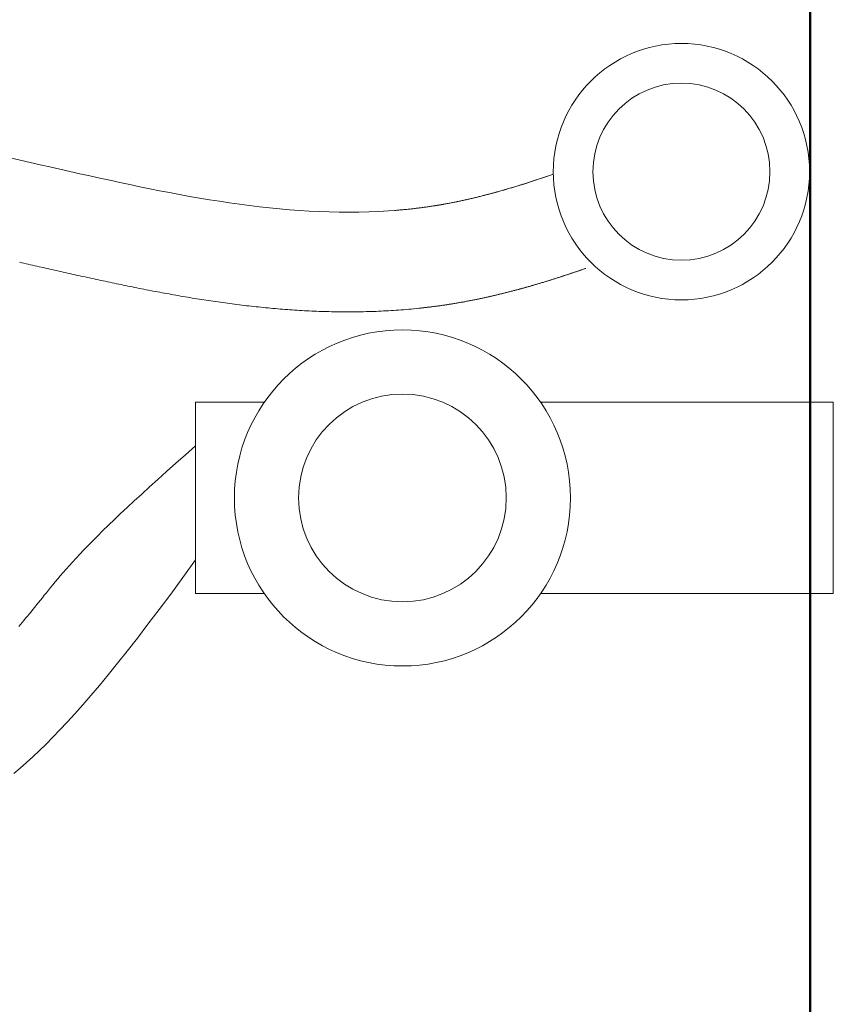
# Model space of a CAD drawing. Units: inches. Extents: x 64 to 1167, y 117 to 939.
# Tile 9 of 56: x 230.36 to 234.443, y 590.326 to 595.266. Entities that reach past the tile are written whole.
import ezdxf

# ---------------------------------------------------------------- set-up
doc = ezdxf.new("R2010")
doc.units = ezdxf.units.IN
doc.header["$MEASUREMENT"] = 0
doc.layers.add('A-FLOR-FIXT', color=8, linetype='Continuous', lineweight=18)
doc.layers.add('A-WALL', color=7, linetype='Continuous', lineweight=50)

# ---------------------------------------------------------------- blocks, each defined once
blk = doc.blocks.new('FAUCET')
for points in [[(1.4695, 2.7601), (0.0003, 2.7601), (0.0003, 1.7995), (1.4695, 1.7995)], [(2.8559, 1.7995), (3.2005, 1.7995), (3.2005, 2.7601), (2.8559, 2.7601)]]:
    blk.add_lwpolyline(points)
for points in [[(3.2005, 2.5912, 0), (3.2645, 2.6791, 0), (3.3257, 2.762, 0), (3.384, 2.8402, 0), (3.4397, 2.9138, 0), (3.493, 2.9831, 0), (3.5438, 3.0482, 0), (3.5924, 3.1094, 0), (3.639, 3.1668, 0), (3.6835, 3.2206, 0), (3.7262, 3.2711, 0), (3.7672, 3.3184, 0), (3.8067, 3.3628, 0), (3.8447, 3.4044, 0), (3.8814, 3.4435, 0), (3.9169, 3.4802, 0), (3.9514, 3.5148, 0), (3.985, 3.5473, 0), (4.0178, 3.5782, 0), (4.05, 3.6075, 0), (4.0816, 3.6354, 0), (4.1129, 3.6621, 0)], [(4.131, 0.5741, 0), (4.0812, 0.5853, 0), (4.0315, 0.5965, 0), (3.9816, 0.6078, 0), (3.9318, 0.6191, 0), (3.8819, 0.6304, 0), (3.8319, 0.6417, 0), (3.7819, 0.6529, 0), (3.7319, 0.6641, 0), (3.6819, 0.6752, 0), (3.6318, 0.6862, 0), (3.5817, 0.697, 0), (3.5316, 0.7077, 0), (3.4815, 0.7182, 0), (3.4313, 0.7284, 0), (3.3812, 0.7384, 0), (3.331, 0.7481, 0), (3.2809, 0.7575, 0), (3.2307, 0.7666, 0), (3.1806, 0.7753, 0), (3.1304, 0.7837, 0), (3.0803, 0.7916, 0), (3.0302, 0.7991, 0), (2.9801, 0.8062, 0), (2.93, 0.8128, 0), (2.88, 0.8188, 0), (2.83, 0.8244, 0), (2.78, 0.8293, 0), (2.73, 0.8337, 0), (2.6801, 0.8375, 0), (2.6302, 0.8406, 0), (2.5804, 0.8431, 0), (2.5307, 0.8449, 0), (2.4809, 0.846, 0), (2.4313, 0.8463, 0), (2.3817, 0.8458, 0), (2.3321, 0.8446, 0), (2.2827, 0.8426, 0), (2.2333, 0.8397, 0), (2.1839, 0.8359, 0), (2.1347, 0.8312, 0), (2.0855, 0.8256, 0), (2.0364, 0.8191, 0), (1.9874, 0.8116, 0), (1.9385, 0.8031, 0), (1.8897, 0.7936, 0), (1.8409, 0.7831, 0), (1.7923, 0.7717, 0), (1.7437, 0.7595, 0), (1.6952, 0.7465, 0), (1.6468, 0.7328, 0), (1.5984, 0.7185, 0), (1.55, 0.7035, 0), (1.5018, 0.6879, 0), (1.4535, 0.6719, 0), (1.4054, 0.6555, 0)], [(3.2005, 2.0185, 0), (3.2517, 2.0633, 0), (3.3003, 2.1062, 0), (3.3465, 2.1473, 0), (3.3904, 2.1866, 0), (3.4319, 2.2242, 0), (3.4713, 2.2602, 0), (3.5085, 2.2945, 0), (3.5437, 2.3273, 0), (3.5769, 2.3586, 0), (3.6083, 2.3884, 0), (3.6378, 2.4169, 0), (3.6656, 2.444, 0), (3.6917, 2.4699, 0), (3.7163, 2.4945, 0), (3.7394, 2.518, 0), (3.761, 2.5404, 0), (3.7814, 2.5617, 0), (3.8004, 2.582, 0), (3.8183, 2.6014, 0), (3.8351, 2.6199, 0), (3.8509, 2.6376, 0), (3.8657, 2.6545, 0), (3.8797, 2.6707, 0), (3.8929, 2.6862, 0), (3.9054, 2.7011, 0), (3.9172, 2.7154, 0), (3.9286, 2.7293, 0), (3.9394, 2.7427, 0), (3.9499, 2.7557, 0), (3.96, 2.7684, 0), (3.9699, 2.7808, 0), (3.9797, 2.7931, 0), (3.9893, 2.8051, 0), (3.9989, 2.8169, 0), (4.0083, 2.8285, 0), (4.0176, 2.84, 0), (4.0268, 2.8512, 0), (4.0359, 2.8623, 0), (4.0449, 2.8732, 0), (4.0538, 2.8839, 0), (4.0625, 2.8945, 0), (4.0712, 2.9048, 0), (4.0798, 2.9151, 0), (4.0883, 2.9251, 0)], [(4.0838, 1.0975, 0), (4.073, 1.0999, 0), (4.0622, 1.1023, 0), (4.0514, 1.1048, 0), (4.0406, 1.1072, 0), (4.0298, 1.1097, 0), (4.0189, 1.1121, 0), (4.0081, 1.1146, 0), (3.9972, 1.117, 0), (3.9863, 1.1195, 0), (3.9754, 1.1219, 0), (3.9645, 1.1244, 0), (3.9536, 1.1269, 0), (3.9426, 1.1293, 0), (3.9317, 1.1318, 0), (3.9207, 1.1342, 0), (3.9097, 1.1367, 0), (3.8988, 1.1392, 0), (3.8878, 1.1416, 0), (3.8767, 1.1441, 0), (3.8657, 1.1466, 0), (3.8547, 1.149, 0), (3.8437, 1.1515, 0), (3.8326, 1.154, 0), (3.8215, 1.1564, 0), (3.8104, 1.1589, 0), (3.7994, 1.1614, 0), (3.7883, 1.1638, 0), (3.7771, 1.1663, 0), (3.766, 1.1687, 0), (3.7549, 1.1712, 0), (3.7437, 1.1736, 0), (3.7325, 1.1761, 0), (3.7214, 1.1785, 0), (3.7102, 1.1809, 0), (3.699, 1.1834, 0), (3.6878, 1.1858, 0), (3.6765, 1.1882, 0), (3.6653, 1.1906, 0), (3.654, 1.193, 0), (3.6428, 1.1954, 0), (3.6315, 1.1978, 0), (3.6202, 1.2002, 0), (3.6089, 1.2026, 0), (3.5976, 1.205, 0), (3.5863, 1.2073, 0), (3.5749, 1.2097, 0), (3.5636, 1.212, 0), (3.5522, 1.2144, 0), (3.5409, 1.2167, 0), (3.5295, 1.219, 0), (3.5181, 1.2213, 0), (3.5067, 1.2236, 0), (3.4953, 1.2259, 0), (3.4838, 1.2282, 0), (3.4724, 1.2304, 0), (3.4609, 1.2327, 0), (3.4495, 1.2349, 0), (3.438, 1.2371, 0), (3.4265, 1.2394, 0), (3.415, 1.2416, 0), (3.4035, 1.2438, 0), (3.392, 1.2459, 0), (3.3804, 1.2481, 0), (3.3689, 1.2502, 0), (3.3573, 1.2524, 0), (3.3457, 1.2545, 0), (3.3342, 1.2566, 0), (3.3226, 1.2587, 0), (3.311, 1.2607, 0), (3.2993, 1.2628, 0), (3.2877, 1.2648, 0), (3.2761, 1.2669, 0), (3.2644, 1.2689, 0), (3.2527, 1.2708, 0), (3.2411, 1.2728, 0), (3.2294, 1.2748, 0), (3.2177, 1.2767, 0), (3.206, 1.2786, 0), (3.1942, 1.2805, 0), (3.1825, 1.2824, 0), (3.1708, 1.2842, 0), (3.159, 1.2861, 0), (3.1472, 1.2879, 0), (3.1354, 1.2897, 0), (3.1236, 1.2914, 0), (3.1118, 1.2932, 0), (3.1, 1.2949, 0), (3.0882, 1.2966, 0), (3.0764, 1.2983, 0), (3.0645, 1.2999, 0), (3.0526, 1.3016, 0), (3.0408, 1.3032, 0), (3.0289, 1.3048, 0), (3.017, 1.3063, 0), (3.0051, 1.3079, 0), (2.9932, 1.3094, 0), (2.9812, 1.3109, 0), (2.9693, 1.3123, 0), (2.9573, 1.3138, 0), (2.9454, 1.3152, 0), (2.9334, 1.3166, 0), (2.9214, 1.3179, 0), (2.9094, 1.3193, 0), (2.8974, 1.3206, 0), (2.8854, 1.3218, 0), (2.8733, 1.3231, 0), (2.8613, 1.3243, 0), (2.8492, 1.3255, 0), (2.8372, 1.3266, 0), (2.8251, 1.3278, 0), (2.813, 1.3289, 0), (2.8009, 1.3299, 0), (2.7888, 1.331, 0), (2.7767, 1.332, 0), (2.7645, 1.333, 0), (2.7524, 1.3339, 0), (2.7402, 1.3348, 0), (2.7281, 1.3357, 0), (2.7159, 1.3365, 0), (2.7037, 1.3374, 0), (2.6915, 1.3381, 0), (2.6793, 1.3389, 0), (2.6671, 1.3396, 0), (2.6548, 1.3403, 0), (2.6426, 1.3409, 0), (2.6303, 1.3415, 0), (2.6181, 1.3421, 0), (2.6058, 1.3427, 0), (2.5935, 1.3432, 0), (2.5812, 1.3436, 0), (2.5689, 1.3441, 0), (2.5566, 1.3445, 0), (2.5442, 1.3448, 0), (2.5319, 1.3451, 0), (2.5195, 1.3454, 0), (2.5072, 1.3457, 0), (2.4948, 1.3459, 0), (2.4824, 1.346, 0), (2.47, 1.3462, 0), (2.4576, 1.3462, 0), (2.4452, 1.3463, 0), (2.4328, 1.3463, 0), (2.4203, 1.3463, 0), (2.4079, 1.3462, 0), (2.3954, 1.3461, 0), (2.3829, 1.3459, 0), (2.3704, 1.3457, 0), (2.3579, 1.3455, 0), (2.3454, 1.3452, 0), (2.3329, 1.3449, 0), (2.3204, 1.3445, 0), (2.3079, 1.3441, 0), (2.2953, 1.3436, 0), (2.2828, 1.3431, 0), (2.2702, 1.3425, 0), (2.2576, 1.3419, 0), (2.2451, 1.3413, 0), (2.2325, 1.3406, 0), (2.2199, 1.3398, 0), (2.2073, 1.339, 0), (2.1946, 1.3382, 0), (2.182, 1.3373, 0), (2.1694, 1.3363, 0), (2.1567, 1.3354, 0), (2.1441, 1.3343, 0), (2.1314, 1.3332, 0), (2.1188, 1.3321, 0), (2.1061, 1.3309, 0), (2.0934, 1.3296, 0), (2.0807, 1.3283, 0), (2.068, 1.327, 0), (2.0553, 1.3255, 0), (2.0426, 1.3241, 0), (2.0299, 1.3226, 0), (2.0172, 1.321, 0), (2.0045, 1.3194, 0), (1.9917, 1.3177, 0), (1.979, 1.3159, 0), (1.9662, 1.3141, 0), (1.9535, 1.3123, 0), (1.9407, 1.3104, 0), (1.9279, 1.3084, 0), (1.9152, 1.3064, 0), (1.9024, 1.3043, 0), (1.8896, 1.3022, 0), (1.8769, 1.3, 0), (1.8642, 1.2977, 0), (1.8515, 1.2954, 0), (1.8388, 1.2931, 0), (1.8262, 1.2907, 0), (1.8136, 1.2882, 0), (1.801, 1.2857, 0), (1.7884, 1.2832, 0), (1.7759, 1.2806, 0), (1.7634, 1.2779, 0), (1.7509, 1.2752, 0), (1.7385, 1.2725, 0), (1.726, 1.2697, 0), (1.7137, 1.2669, 0), (1.7013, 1.264, 0), (1.689, 1.2611, 0), (1.6767, 1.2582, 0), (1.6644, 1.2552, 0), (1.6521, 1.2521, 0), (1.6399, 1.2491, 0), (1.6277, 1.246, 0), (1.6156, 1.2428, 0), (1.6034, 1.2396, 0), (1.5913, 1.2364, 0), (1.5792, 1.2332, 0), (1.5672, 1.2299, 0), (1.5552, 1.2266, 0), (1.5432, 1.2232, 0), (1.5312, 1.2199, 0), (1.5193, 1.2165, 0), (1.5074, 1.213, 0), (1.4955, 1.2096, 0), (1.4837, 1.2061, 0), (1.4719, 1.2026, 0), (1.4601, 1.199, 0), (1.4483, 1.1954, 0), (1.4366, 1.1919, 0), (1.4249, 1.1882, 0), (1.4133, 1.1846, 0), (1.4016, 1.181, 0), (1.39, 1.1773, 0), (1.3784, 1.1736, 0), (1.3669, 1.1699, 0), (1.3554, 1.1661, 0), (1.3439, 1.1624, 0), (1.3325, 1.1586, 0), (1.321, 1.1548, 0), (1.3097, 1.151, 0), (1.2983, 1.1472, 0), (1.287, 1.1434, 0), (1.2757, 1.1396, 0), (1.2644, 1.1357, 0), (1.2532, 1.1319, 0), (1.242, 1.128, 0)], [(2.0792, 1.3282, 0), (2.0747, 1.3277, 0), (2.0701, 1.3272, 0), (2.0655, 1.3267, 0), (2.0609, 1.3262, 0), (2.0563, 1.3257, 0), (2.0518, 1.3251, 0), (2.0472, 1.3246, 0), (2.0426, 1.3241, 0), (2.038, 1.3235, 0), (2.0334, 1.323, 0), (2.0288, 1.3224, 0), (2.0242, 1.3219, 0), (2.0197, 1.3213, 0), (2.0151, 1.3207, 0), (2.0105, 1.3201, 0), (2.0059, 1.3195, 0), (2.0013, 1.3189, 0), (1.9967, 1.3183, 0), (1.9921, 1.3177, 0), (1.9875, 1.3171, 0), (1.9829, 1.3165, 0), (1.9783, 1.3159, 0), (1.9737, 1.3152, 0), (1.9691, 1.3146, 0), (1.9645, 1.3139, 0), (1.9599, 1.3132, 0), (1.9553, 1.3126, 0), (1.9507, 1.3119, 0), (1.9461, 1.3112, 0), (1.9415, 1.3105, 0), (1.9369, 1.3098, 0), (1.9323, 1.3091, 0), (1.9277, 1.3084, 0), (1.9231, 1.3077, 0), (1.9185, 1.3069, 0), (1.9139, 1.3062, 0), (1.9093, 1.3054, 0), (1.9047, 1.3047, 0), (1.9001, 1.3039, 0), (1.8955, 1.3032, 0), (1.8909, 1.3024, 0), (1.8863, 1.3016, 0), (1.8817, 1.3008, 0), (1.8771, 1.3, 0), (1.8725, 1.2992, 0), (1.8679, 1.2984, 0), (1.8633, 1.2976, 0), (1.8587, 1.2968, 0), (1.8541, 1.2959, 0), (1.8496, 1.2951, 0), (1.845, 1.2943, 0), (1.8404, 1.2934, 0), (1.8359, 1.2925, 0), (1.8313, 1.2917, 0), (1.8268, 1.2908, 0), (1.8222, 1.2899, 0), (1.8177, 1.289, 0), (1.8131, 1.2882, 0), (1.8086, 1.2873, 0), (1.804, 1.2863, 0), (1.7995, 1.2854, 0), (1.795, 1.2845, 0), (1.7904, 1.2836, 0), (1.7859, 1.2827, 0), (1.7814, 1.2817, 0), (1.7769, 1.2808, 0), (1.7724, 1.2798, 0), (1.7679, 1.2789, 0), (1.7634, 1.2779, 0), (1.7589, 1.277, 0), (1.7544, 1.276, 0), (1.7499, 1.275, 0), (1.7454, 1.274, 0), (1.7409, 1.273, 0), (1.7364, 1.272, 0), (1.7319, 1.271, 0), (1.7275, 1.27, 0), (1.723, 1.269, 0), (1.7185, 1.268, 0), (1.714, 1.267, 0), (1.7096, 1.266, 0), (1.7051, 1.2649, 0), (1.7007, 1.2639, 0), (1.6962, 1.2628, 0), (1.6918, 1.2618, 0), (1.6873, 1.2607, 0), (1.6829, 1.2597, 0), (1.6785, 1.2586, 0), (1.674, 1.2575, 0), (1.6696, 1.2564, 0), (1.6652, 1.2554, 0), (1.6607, 1.2543, 0), (1.6563, 1.2532, 0), (1.6519, 1.2521, 0), (1.6475, 1.251, 0), (1.6431, 1.2499, 0), (1.6387, 1.2488, 0), (1.6343, 1.2476, 0), (1.6299, 1.2465, 0), (1.6255, 1.2454, 0), (1.6211, 1.2443, 0), (1.6167, 1.2431, 0), (1.6124, 1.242, 0), (1.608, 1.2408, 0), (1.6036, 1.2397, 0), (1.5992, 1.2385, 0), (1.5949, 1.2374, 0), (1.5905, 1.2362, 0), (1.5862, 1.235, 0), (1.5818, 1.2339, 0), (1.5774, 1.2327, 0), (1.5731, 1.2315, 0), (1.5688, 1.2303, 0), (1.5644, 1.2291, 0), (1.5601, 1.2279, 0), (1.5558, 1.2267, 0), (1.5514, 1.2255, 0), (1.5471, 1.2243, 0), (1.5428, 1.2231, 0), (1.5385, 1.2219, 0), (1.5342, 1.2207, 0), (1.5298, 1.2195, 0), (1.5255, 1.2182, 0), (1.5212, 1.217, 0), (1.5169, 1.2158, 0), (1.5126, 1.2145, 0), (1.5084, 1.2133, 0), (1.5041, 1.2121, 0), (1.4998, 1.2108, 0), (1.4955, 1.2096, 0), (1.4912, 1.2083, 0), (1.487, 1.207, 0), (1.4827, 1.2058, 0), (1.4784, 1.2045, 0), (1.4742, 1.2032, 0), (1.4699, 1.202, 0), (1.4657, 1.2007, 0), (1.4614, 1.1994, 0), (1.4572, 1.1981, 0), (1.4529, 1.1969, 0), (1.4487, 1.1956, 0), (1.4445, 1.1943, 0), (1.4403, 1.193, 0), (1.436, 1.1917, 0), (1.4318, 1.1904, 0), (1.4276, 1.1891, 0), (1.4234, 1.1878, 0), (1.4192, 1.1865, 0), (1.415, 1.1851, 0), (1.4108, 1.1838, 0), (1.4066, 1.1825, 0), (1.4024, 1.1812, 0), (1.3982, 1.1799, 0), (1.394, 1.1785, 0), (1.3898, 1.1772, 0), (1.3856, 1.1759, 0), (1.3815, 1.1746, 0), (1.3773, 1.1732, 0), (1.3731, 1.1719, 0), (1.369, 1.1705, 0), (1.3648, 1.1692, 0), (1.3607, 1.1678, 0), (1.3565, 1.1665, 0), (1.3524, 1.1652, 0), (1.3482, 1.1638, 0), (1.3441, 1.1624, 0), (1.34, 1.1611, 0), (1.3358, 1.1597, 0), (1.3317, 1.1584, 0), (1.3276, 1.157, 0), (1.3235, 1.1556, 0), (1.3194, 1.1543, 0), (1.3153, 1.1529, 0), (1.3112, 1.1515, 0), (1.307, 1.1502, 0), (1.303, 1.1488, 0), (1.2989, 1.1474, 0), (1.2948, 1.146, 0), (1.2907, 1.1447, 0), (1.2866, 1.1433, 0), (1.2825, 1.1419, 0), (1.2785, 1.1405, 0), (1.2744, 1.1391, 0), (1.2703, 1.1378, 0), (1.2663, 1.1364, 0), (1.2622, 1.135, 0), (1.2582, 1.1336, 0), (1.2541, 1.1322, 0), (1.2501, 1.1308, 0), (1.246, 1.1294, 0), (1.242, 1.128, 0)], [(2.2006, 0.8373, 0), (2.1956, 0.8369, 0), (2.1905, 0.8364, 0), (2.1854, 0.836, 0), (2.1804, 0.8356, 0), (2.1753, 0.8351, 0), (2.1702, 0.8347, 0), (2.1652, 0.8342, 0), (2.1601, 0.8337, 0), (2.155, 0.8333, 0), (2.15, 0.8328, 0), (2.1449, 0.8323, 0), (2.1399, 0.8318, 0), (2.1348, 0.8312, 0), (2.1298, 0.8307, 0), (2.1247, 0.8302, 0), (2.1196, 0.8296, 0), (2.1146, 0.8291, 0), (2.1095, 0.8285, 0), (2.1045, 0.8279, 0), (2.0994, 0.8273, 0), (2.0944, 0.8267, 0), (2.0893, 0.8261, 0), (2.0843, 0.8255, 0), (2.0792, 0.8249, 0), (2.0742, 0.8242, 0), (2.0691, 0.8236, 0), (2.0641, 0.8229, 0), (2.059, 0.8222, 0), (2.054, 0.8216, 0), (2.049, 0.8209, 0), (2.0439, 0.8202, 0), (2.0389, 0.8194, 0), (2.0338, 0.8187, 0), (2.0288, 0.818, 0), (2.0238, 0.8173, 0), (2.0187, 0.8165, 0), (2.0137, 0.8157, 0), (2.0087, 0.815, 0), (2.0036, 0.8142, 0), (1.9986, 0.8134, 0), (1.9936, 0.8126, 0), (1.9885, 0.8118, 0), (1.9835, 0.8109, 0), (1.9785, 0.8101, 0), (1.9734, 0.8093, 0), (1.9684, 0.8084, 0), (1.9634, 0.8075, 0), (1.9583, 0.8067, 0), (1.9533, 0.8058, 0), (1.9483, 0.8049, 0), (1.9433, 0.8039, 0), (1.9383, 0.803, 0), (1.9332, 0.8021, 0), (1.9282, 0.8012, 0), (1.9232, 0.8002, 0), (1.9182, 0.7992, 0), (1.9132, 0.7983, 0), (1.9081, 0.7973, 0), (1.9031, 0.7963, 0), (1.8981, 0.7953, 0), (1.8931, 0.7943, 0), (1.8881, 0.7932, 0), (1.8831, 0.7922, 0), (1.8781, 0.7911, 0), (1.8731, 0.7901, 0), (1.868, 0.789, 0), (1.863, 0.788, 0), (1.858, 0.7869, 0), (1.853, 0.7858, 0), (1.848, 0.7847, 0), (1.843, 0.7836, 0), (1.838, 0.7824, 0), (1.833, 0.7813, 0), (1.828, 0.7802, 0), (1.823, 0.779, 0), (1.818, 0.7778, 0), (1.813, 0.7767, 0), (1.808, 0.7755, 0), (1.803, 0.7743, 0), (1.798, 0.7731, 0), (1.793, 0.7719, 0), (1.788, 0.7707, 0), (1.783, 0.7695, 0), (1.778, 0.7682, 0), (1.773, 0.767, 0), (1.768, 0.7657, 0), (1.7631, 0.7645, 0), (1.7581, 0.7632, 0), (1.7531, 0.7619, 0), (1.7481, 0.7607, 0), (1.7431, 0.7594, 0), (1.7381, 0.7581, 0), (1.7331, 0.7568, 0), (1.7281, 0.7554, 0), (1.7232, 0.7541, 0), (1.7182, 0.7528, 0), (1.7132, 0.7514, 0), (1.7082, 0.7501, 0), (1.7032, 0.7487, 0), (1.6982, 0.7474, 0), (1.6933, 0.746, 0), (1.6883, 0.7446, 0), (1.6833, 0.7432, 0), (1.6783, 0.7418, 0), (1.6733, 0.7404, 0), (1.6684, 0.739, 0), (1.6634, 0.7376, 0), (1.6584, 0.7362, 0), (1.6534, 0.7348, 0), (1.6485, 0.7333, 0), (1.6435, 0.7319, 0), (1.6385, 0.7304, 0), (1.6335, 0.729, 0), (1.6286, 0.7275, 0), (1.6236, 0.726, 0), (1.6186, 0.7245, 0), (1.6136, 0.7231, 0), (1.6087, 0.7216, 0), (1.6037, 0.7201, 0), (1.5987, 0.7186, 0), (1.5938, 0.7171, 0), (1.5888, 0.7155, 0), (1.5838, 0.714, 0), (1.5789, 0.7125, 0), (1.5739, 0.7109, 0), (1.5689, 0.7094, 0), (1.564, 0.7078, 0), (1.559, 0.7063, 0), (1.554, 0.7047, 0), (1.5491, 0.7032, 0), (1.5441, 0.7016, 0), (1.5392, 0.7, 0), (1.5342, 0.6984, 0), (1.5292, 0.6968, 0), (1.5243, 0.6952, 0), (1.5193, 0.6936, 0), (1.5144, 0.692, 0), (1.5094, 0.6904, 0), (1.5044, 0.6888, 0), (1.4995, 0.6872, 0), (1.4945, 0.6856, 0), (1.4896, 0.6839, 0), (1.4846, 0.6823, 0), (1.4796, 0.6807, 0), (1.4747, 0.679, 0), (1.4697, 0.6774, 0), (1.4648, 0.6757, 0), (1.4598, 0.674, 0), (1.4549, 0.6724, 0), (1.4499, 0.6707, 0), (1.445, 0.669, 0), (1.44, 0.6673, 0), (1.4351, 0.6657, 0), (1.4301, 0.664, 0), (1.4252, 0.6623, 0), (1.4202, 0.6606, 0), (1.4153, 0.6589, 0), (1.4103, 0.6572, 0), (1.4054, 0.6555, 0)], [(2.2006, 0.8373, 0), (2.1956, 0.8369, 0), (2.1905, 0.8364, 0), (2.1854, 0.836, 0), (2.1804, 0.8356, 0), (2.1753, 0.8351, 0), (2.1702, 0.8347, 0), (2.1652, 0.8342, 0), (2.1601, 0.8337, 0), (2.155, 0.8333, 0), (2.15, 0.8328, 0), (2.1449, 0.8323, 0), (2.1399, 0.8318, 0), (2.1348, 0.8312, 0), (2.1298, 0.8307, 0), (2.1247, 0.8302, 0), (2.1196, 0.8296, 0), (2.1146, 0.8291, 0), (2.1095, 0.8285, 0), (2.1045, 0.8279, 0), (2.0994, 0.8273, 0), (2.0944, 0.8267, 0), (2.0893, 0.8261, 0), (2.0843, 0.8255, 0), (2.0792, 0.8249, 0), (2.0742, 0.8242, 0), (2.0691, 0.8236, 0), (2.0641, 0.8229, 0), (2.059, 0.8222, 0), (2.054, 0.8216, 0), (2.049, 0.8209, 0), (2.0439, 0.8202, 0), (2.0389, 0.8194, 0), (2.0338, 0.8187, 0), (2.0288, 0.818, 0), (2.0238, 0.8173, 0), (2.0187, 0.8165, 0), (2.0137, 0.8157, 0), (2.0087, 0.815, 0), (2.0036, 0.8142, 0), (1.9986, 0.8134, 0), (1.9936, 0.8126, 0), (1.9885, 0.8118, 0), (1.9835, 0.8109, 0), (1.9785, 0.8101, 0), (1.9734, 0.8093, 0), (1.9684, 0.8084, 0), (1.9634, 0.8075, 0), (1.9583, 0.8067, 0), (1.9533, 0.8058, 0), (1.9483, 0.8049, 0), (1.9433, 0.8039, 0), (1.9383, 0.803, 0), (1.9332, 0.8021, 0), (1.9282, 0.8012, 0), (1.9232, 0.8002, 0), (1.9182, 0.7992, 0), (1.9132, 0.7983, 0), (1.9081, 0.7973, 0), (1.9031, 0.7963, 0), (1.8981, 0.7953, 0), (1.8931, 0.7943, 0), (1.8881, 0.7932, 0), (1.8831, 0.7922, 0), (1.8781, 0.7911, 0), (1.8731, 0.7901, 0), (1.868, 0.789, 0), (1.863, 0.788, 0), (1.858, 0.7869, 0), (1.853, 0.7858, 0), (1.848, 0.7847, 0), (1.843, 0.7836, 0), (1.838, 0.7824, 0), (1.833, 0.7813, 0), (1.828, 0.7802, 0), (1.823, 0.779, 0), (1.818, 0.7778, 0), (1.813, 0.7767, 0), (1.808, 0.7755, 0), (1.803, 0.7743, 0), (1.798, 0.7731, 0), (1.793, 0.7719, 0), (1.788, 0.7707, 0), (1.783, 0.7695, 0), (1.778, 0.7682, 0), (1.773, 0.767, 0), (1.768, 0.7657, 0), (1.7631, 0.7645, 0), (1.7581, 0.7632, 0), (1.7531, 0.7619, 0), (1.7481, 0.7607, 0), (1.7431, 0.7594, 0), (1.7381, 0.7581, 0), (1.7331, 0.7568, 0), (1.7281, 0.7554, 0), (1.7232, 0.7541, 0), (1.7182, 0.7528, 0), (1.7132, 0.7514, 0), (1.7082, 0.7501, 0), (1.7032, 0.7487, 0), (1.6982, 0.7474, 0), (1.6933, 0.746, 0), (1.6883, 0.7446, 0), (1.6833, 0.7432, 0), (1.6783, 0.7418, 0), (1.6733, 0.7404, 0), (1.6684, 0.739, 0), (1.6634, 0.7376, 0), (1.6584, 0.7362, 0), (1.6534, 0.7348, 0), (1.6485, 0.7333, 0), (1.6435, 0.7319, 0), (1.6385, 0.7304, 0), (1.6335, 0.729, 0), (1.6286, 0.7275, 0), (1.6236, 0.726, 0), (1.6186, 0.7245, 0), (1.6136, 0.7231, 0), (1.6087, 0.7216, 0), (1.6037, 0.7201, 0), (1.5987, 0.7186, 0), (1.5938, 0.7171, 0), (1.5888, 0.7155, 0), (1.5838, 0.714, 0), (1.5789, 0.7125, 0), (1.5739, 0.7109, 0), (1.5689, 0.7094, 0), (1.564, 0.7078, 0), (1.559, 0.7063, 0), (1.554, 0.7047, 0), (1.5491, 0.7032, 0), (1.5441, 0.7016, 0), (1.5392, 0.7, 0), (1.5342, 0.6984, 0), (1.5292, 0.6968, 0), (1.5243, 0.6952, 0), (1.5193, 0.6936, 0), (1.5144, 0.692, 0), (1.5094, 0.6904, 0), (1.5044, 0.6888, 0), (1.4995, 0.6872, 0), (1.4945, 0.6856, 0), (1.4896, 0.6839, 0), (1.4846, 0.6823, 0), (1.4796, 0.6807, 0), (1.4747, 0.679, 0), (1.4697, 0.6774, 0), (1.4648, 0.6757, 0), (1.4598, 0.674, 0), (1.4549, 0.6724, 0), (1.4499, 0.6707, 0), (1.445, 0.669, 0), (1.44, 0.6673, 0), (1.4351, 0.6657, 0), (1.4301, 0.664, 0), (1.4252, 0.6623, 0), (1.4202, 0.6606, 0), (1.4153, 0.6589, 0), (1.4103, 0.6572, 0), (1.4054, 0.6555, 0)]]:
    blk.add_polyline3d(points)
for centre, radius in [((2.1627, 2.2798), 0.8433), ((2.1627, 2.2798), 0.5212), ((0.7624, 0.6428), 0.6431), ((0.7624, 0.6428), 0.4442)]:
    blk.add_circle(centre, radius)

msp = doc.modelspace()

# ---------------------------------------------------------------- linework, layer by layer
at = {"layer": 'A-WALL'}
msp.add_line((234.3263, 633.1998), (234.3263, 585.1998), dxfattribs=at)

# ---------------------------------------------------------------- block references
at = {"layer": 'A-FLOR-FIXT', "rotation": 180}
msp.add_blockref('FAUCET', (234.4434, 595.1462), dxfattribs=at)

doc.saveas('drawing.dxf')
